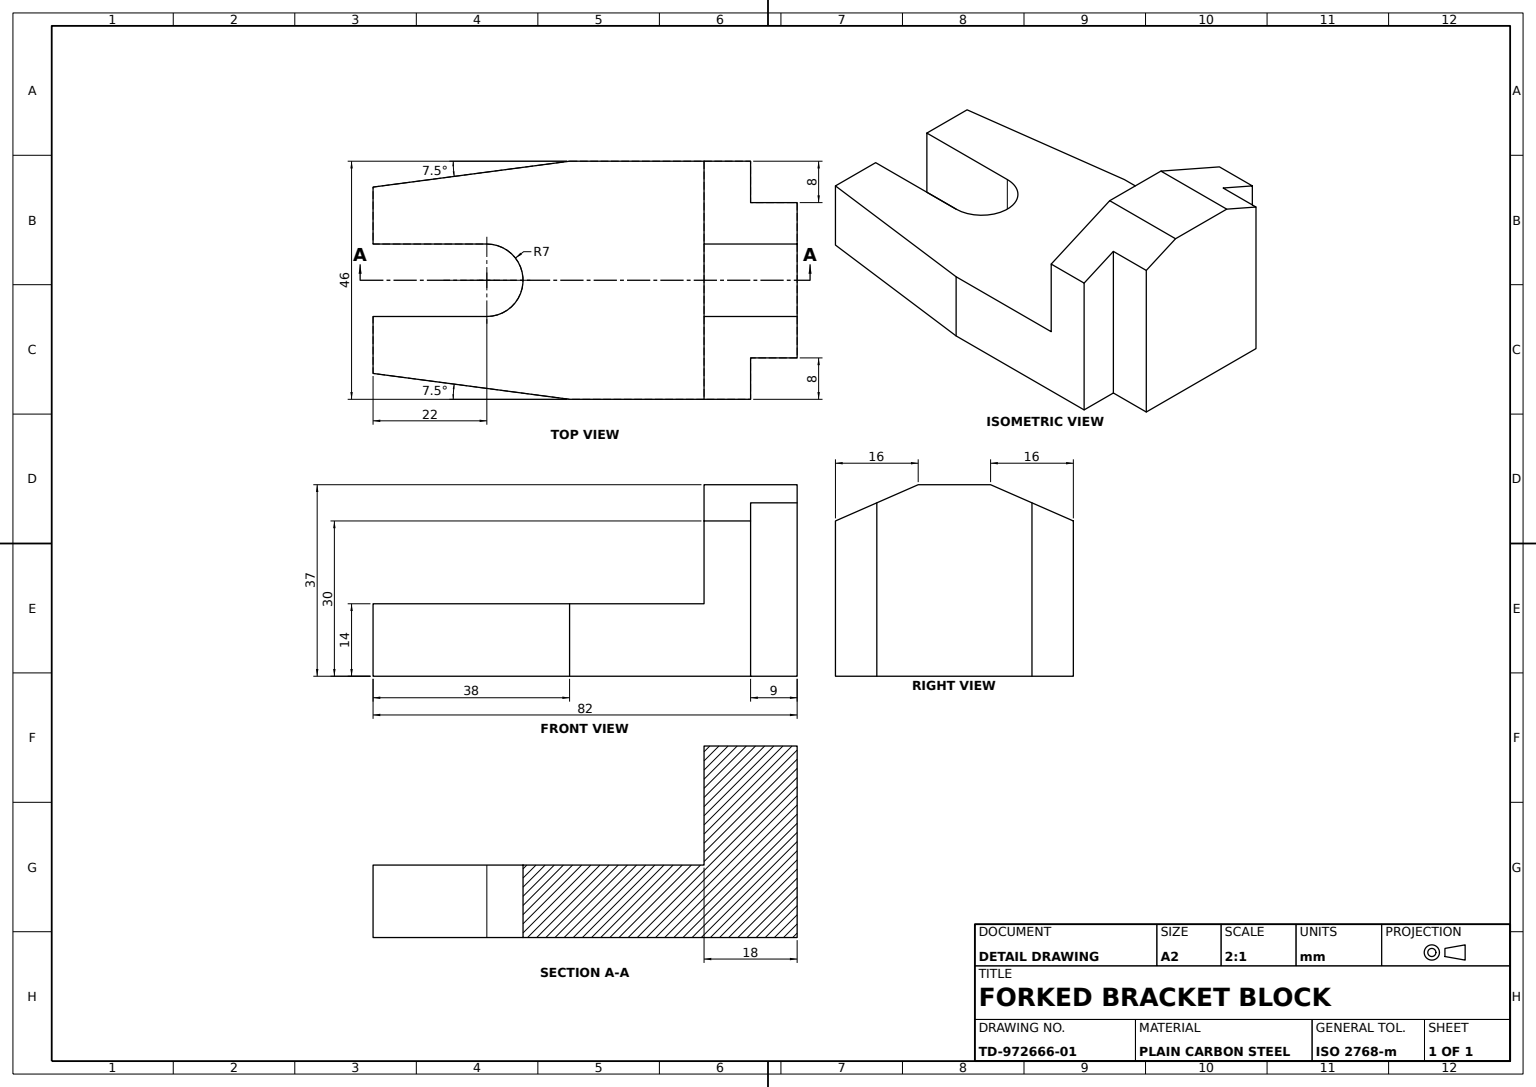
SolidWorks part; units mm, degrees
material "Plain Carbon Steel"
ref_plane "Front Plane" through (0, 0, 0) normal (0, 0, 1) x (1, 0, 0)
ref_plane "Top Plane" through (0, 0, 0) normal (0, 1, 0) x (1, 0, 0)
ref_plane "Right Plane" through (0, 0, 0) normal (1, 0, 0) x (0, 0, -1)
sketch "Base Profile Sketch" plane through (0, 0, 0) normal (0, 0, 1) x (1, 0, 0)
  line L0 (-23, 15) -> (-7, 22)
  line L1 (23, -15) -> (-23, -15)
  line L2 (23, -15) -> (23, 15)
  line L4 (-23, -15) -> (-23, 15)
  line L5 (23, -15) -> (-23, 15) construction
  line L6 (23, 15) -> (-23, -15) construction
  line L7 (-7, 22) -> (7, 22)
  line L8 (7, 22) -> (23, 15)
  point P0 (0, 0)
  point P6 (0, 22)
  dimension "D1" = 14
  dimension "D2" = 16
  dimension "D3" = 46
  dimension "D4" = 7
  dimension "D5" = 30
extrude "Forked Base" add sketch "Base Profile Sketch" along normal blind 18
sketch "Upright Profile Sketch" plane through (0, -15, 0) normal (0, -1, 0) x (-1, 0, 0)
  line L0 (-23, -18) -> (-23, -44)
  line L1 (-23, -44) -> (-18, -82)
  line L2 (-18, -82) -> (-7, -82)
  line L3 (-7, -82) -> (-7, -60)
  line L4 (0, 0) -> (0, -110.1918) construction
  line L5 (7, -82) -> (7, -60)
  line L6 (18, -82) -> (7, -82)
  line L7 (23, -44) -> (18, -82)
  line L8 (23, -18) -> (23, -44)
  line L9 (-23, -18) -> (23, -18)
  arc A0 (7, -60) -> (-7, -60) centre (0, -60) ccw
  dimension "D4" = 14
  dimension "D1" = 26
  dimension "D2" = 38
  dimension "D3" = 11
  dimension "D5" = 22
extrude "Upright Boss" add sketch "Upright Profile Sketch" against normal blind 14
sketch "Notch Sketch 8x9" plane through (0, -15, 0) normal (0, -1, 0) x (1, 0, 0)
  line L1 (23, 0) -> (15, 0)
  line L2 (23, 0) -> (23, 9)
  line L3 (23, 9) -> (15, 9)
  line L4 (15, 0) -> (15, 9)
  dimension "D1" = 8
  dimension "D2" = 9
extrude "Notch Cut 8x9" cut sketch "Notch Sketch 8x9" against normal through all
mirror "Notch Mirror" about plane through (0, 0, 0) normal (1, 0, 0) of "Notch Cut 8x9"
